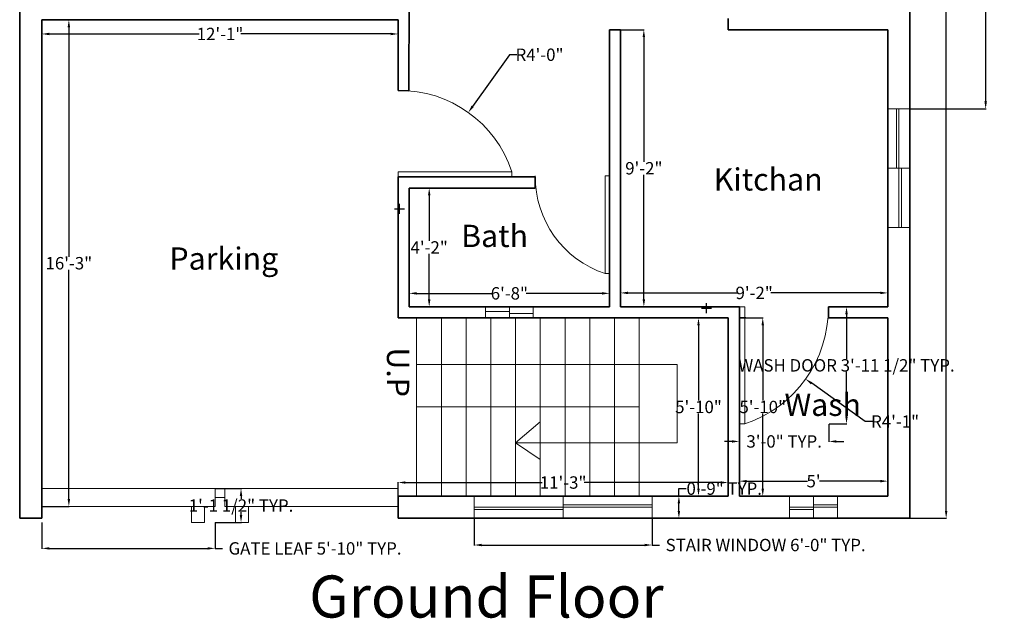
# Model space of a CAD drawing. Units: inches. Extents: x 534 to 1461, y 174 to 793.
# Tile 1 of 4: x 534 to 932, y 174 to 416. Entities that reach past the tile are written whole.
import ezdxf

# ---------------------------------------------------------------- set-up
doc = ezdxf.new("R2010")
doc.units = ezdxf.units.IN
doc.header["$MEASUREMENT"] = 0
for name, color, linetype, lineweight in [('A-ANNO-DIMS', 2, 'Continuous', 13), ('A-ANNO-SYMB', 7, 'Continuous', 15), ('A-FLOR-STRS', 7, 'Continuous', 18), ('A-GLAZ', 6, 'Continuous', 18), ('A-WALL', 7, 'Continuous', 35)]:
    doc.layers.add(name, color=color, linetype=linetype, lineweight=lineweight)
for name, color, linetype, lineweight, true_color in [('A-ANNO-TEXT', 254, 'Continuous', 18, 0xddb3d4), ('A-ANNO-TITL', 32, 'Continuous', 25, 0xcd6928), ('A-AREA-IDEN', 254, 'Continuous', 18, 0xddb3d4), ('A-DOOR', 165, 'Continuous', 20, 0x5e67af)]:
    doc.layers.add(name, color=color, linetype=linetype, lineweight=lineweight, true_color=true_color)
doc.styles.get("Standard").update_dxf_attribs({"font": 'arial.ttf'})
doc.dimstyles.get("Standard").update_dxf_attribs({"dimtxt": 5, "dimasz": 3, "dimexe": 0.18, "dimexo": 0.0625, "dimgap": 0.09, "dimtad": 0, "dimtih": 1, "dimtoh": 1, "dimdec": 1, "dimrnd": 5, "dimzin": 0, "dimdsep": 46, "dimlunit": 4, "dimtxsty": 'Standard', "dimcen": 2, "dimclrd": 4, "dimclrt": 1, "dimadec": 0, "dimazin": 0, "dimtfac": 1, "dimtdec": 1, "dimtofl": 0, "dimtmove": 0, "dimatfit": 3, "dimfxl": 1, "dimtfillclr": 1, "dimtolj": 1, "dimtzin": 0, "dimarcsym": 0})

# ---------------------------------------------------------------- blocks, each defined once
blk = doc.blocks.new('*D13')
at = {"layer": 'A-ANNO-DIMS', "color": 0, "lineweight": -2, "transparency": 16777216}
for p, q in [((691.62, 348), (699.83, 348)), ((699.65, 345), (699.65, 326.6)), ((699.65, 303), (699.65, 321.4)), ((691.62, 300), (699.83, 300))]:
    blk.add_line(p, q, dxfattribs=at)
at = {"layer": 'A-ANNO-DIMS', "color": 0, "transparency": 16777216}
for points in [[(699.15, 345), (700.15, 345), (699.65, 348)], [(699.15, 303), (700.15, 303), (699.65, 300)]]:
    blk.add_solid(points, dxfattribs=at)
at = {"layer": 'Defpoints', "color": 0, "transparency": 16777216}
for p in [(691.56, 348), (691.56, 300), (699.65, 300)]:
    blk.add_point(p, dxfattribs=at)
at = {"layer": 'A-ANNO-DIMS', "color": 0, "transparency": 16777216, "insert": (699.65, 324), "char_height": 5, "attachment_point": 5}
blk.add_mtext('\\A1;4\'-2"', dxfattribs=at)
blk = doc.blocks.new('*D14')
at = {"layer": 'A-ANNO-DIMS', "color": 0, "lineweight": -2, "transparency": 16777216}
for p, q in [((691.56, 300.06), (691.56, 305.62)), ((694.56, 305.44), (725.31, 305.44)), ((769.56, 305.44), (738.81, 305.44)), ((772.56, 300.06), (772.56, 305.62))]:
    blk.add_line(p, q, dxfattribs=at)
at = {"layer": 'A-ANNO-DIMS', "color": 0, "transparency": 16777216}
for points in [[(694.56, 305.94), (694.56, 304.94), (691.56, 305.44)], [(769.56, 305.94), (769.56, 304.94), (772.56, 305.44)]]:
    blk.add_solid(points, dxfattribs=at)
at = {"layer": 'Defpoints', "color": 0, "transparency": 16777216}
for p in [(772.56, 305.44), (691.56, 300), (772.56, 300)]:
    blk.add_point(p, dxfattribs=at)
at = {"layer": 'A-ANNO-DIMS', "color": 0, "transparency": 16777216, "insert": (732.06, 305.44), "char_height": 5, "attachment_point": 5}
blk.add_mtext('\\A1;6\'-8"', dxfattribs=at)
blk = doc.blocks.new('*D15')
at = {"layer": 'A-ANNO-DIMS', "color": 0, "lineweight": -2, "transparency": 16777216}
for p, q in [((777.12, 412), (786.62, 412)), ((786.44, 409), (786.44, 358.64)), ((786.44, 303), (786.44, 353.36)), ((777.12, 300), (786.62, 300))]:
    blk.add_line(p, q, dxfattribs=at)
at = {"layer": 'A-ANNO-DIMS', "color": 0, "transparency": 16777216}
for points in [[(785.94, 409), (786.94, 409), (786.44, 412)], [(785.94, 303), (786.94, 303), (786.44, 300)]]:
    blk.add_solid(points, dxfattribs=at)
at = {"layer": 'Defpoints', "color": 0, "transparency": 16777216}
for p in [(777.06, 412), (777.06, 300), (786.44, 300)]:
    blk.add_point(p, dxfattribs=at)
at = {"layer": 'A-ANNO-DIMS', "color": 0, "transparency": 16777216, "insert": (786.44, 356), "char_height": 5, "attachment_point": 5}
blk.add_mtext('\\A1;9\'-2"', dxfattribs=at)
blk = doc.blocks.new('*D16')
at = {"layer": 'A-ANNO-DIMS', "color": 0, "lineweight": -2, "transparency": 16777216}
for p, q in [((777.06, 300.06), (777.06, 305.79)), ((780.06, 305.61), (824.33, 305.61)), ((882.06, 305.61), (837.8, 305.61)), ((885.06, 300.06), (885.06, 305.79))]:
    blk.add_line(p, q, dxfattribs=at)
at = {"layer": 'A-ANNO-DIMS', "color": 0, "transparency": 16777216}
for points in [[(780.06, 306.11), (780.06, 305.11), (777.06, 305.61)], [(882.06, 306.11), (882.06, 305.11), (885.06, 305.61)]]:
    blk.add_solid(points, dxfattribs=at)
at = {"layer": 'Defpoints', "color": 0, "transparency": 16777216}
for p in [(885.06, 305.61), (777.06, 300), (885.06, 300)]:
    blk.add_point(p, dxfattribs=at)
at = {"layer": 'A-ANNO-DIMS', "color": 0, "transparency": 16777216, "insert": (831.06, 305.61), "char_height": 5, "attachment_point": 5}
blk.add_mtext('\\A1;9\'-2"', dxfattribs=at)
blk = doc.blocks.new('*D17')
at = {"layer": 'A-ANNO-DIMS', "color": 0, "lineweight": -2, "transparency": 16777216}
for p, q in [((825.12, 295.5), (834.7, 295.5)), ((834.52, 292.5), (834.52, 262.14)), ((834.52, 226.5), (834.52, 256.86)), ((825.12, 223.5), (834.7, 223.5))]:
    blk.add_line(p, q, dxfattribs=at)
at = {"layer": 'A-ANNO-DIMS', "color": 0, "transparency": 16777216}
for points in [[(834.02, 292.5), (835.02, 292.5), (834.52, 295.5)], [(834.02, 226.5), (835.02, 226.5), (834.52, 223.5)]]:
    blk.add_solid(points, dxfattribs=at)
at = {"layer": 'Defpoints', "color": 0, "transparency": 16777216}
for p in [(825.06, 295.5), (825.06, 223.5), (834.52, 223.5)]:
    blk.add_point(p, dxfattribs=at)
at = {"layer": 'A-ANNO-DIMS', "color": 0, "transparency": 16777216, "insert": (834.52, 259.5), "char_height": 5, "attachment_point": 5}
blk.add_mtext('\\A1;5\'-10"', dxfattribs=at)
blk = doc.blocks.new('*D18')
at = {"layer": 'A-ANNO-DIMS', "color": 0, "lineweight": -2, "transparency": 16777216}
for p, q in [((825.06, 223.56), (825.06, 229.7)), ((828.06, 229.52), (852.67, 229.52)), ((882.06, 229.52), (857.45, 229.52)), ((885.06, 223.56), (885.06, 229.7))]:
    blk.add_line(p, q, dxfattribs=at)
at = {"layer": 'A-ANNO-DIMS', "color": 0, "transparency": 16777216}
for points in [[(828.06, 230.02), (828.06, 229.02), (825.06, 229.52)], [(882.06, 230.02), (882.06, 229.02), (885.06, 229.52)]]:
    blk.add_solid(points, dxfattribs=at)
at = {"layer": 'Defpoints', "color": 0, "transparency": 16777216}
for p in [(885.06, 229.52), (825.06, 223.5), (885.06, 223.5)]:
    blk.add_point(p, dxfattribs=at)
at = {"layer": 'A-ANNO-DIMS', "color": 0, "transparency": 16777216, "insert": (855.06, 229.52), "char_height": 5, "attachment_point": 5}
blk.add_mtext("\\A1;5'", dxfattribs=at)
blk = doc.blocks.new('*D19')
at = {"layer": 'A-ANNO-DIMS', "color": 0, "lineweight": -2, "transparency": 16777216}
for p, q in [((543.12, 416), (554.12, 416)), ((553.94, 413), (553.94, 320.26)), ((553.94, 222.24), (553.94, 314.97)), ((543.12, 219.24), (554.12, 219.24))]:
    blk.add_line(p, q, dxfattribs=at)
at = {"layer": 'A-ANNO-DIMS', "color": 0, "transparency": 16777216}
for points in [[(553.44, 413), (554.44, 413), (553.94, 416)], [(553.44, 222.24), (554.44, 222.24), (553.94, 219.24)]]:
    blk.add_solid(points, dxfattribs=at)
at = {"layer": 'Defpoints', "color": 0, "transparency": 16777216}
for p in [(543.06, 416), (543.06, 219.24), (553.94, 219.24)]:
    blk.add_point(p, dxfattribs=at)
at = {"layer": 'A-ANNO-DIMS', "color": 0, "transparency": 16777216, "insert": (553.94, 317.62), "char_height": 5, "attachment_point": 5}
blk.add_mtext('\\A1;16\'-3"', dxfattribs=at)
blk = doc.blocks.new('*D20')
at = {"layer": 'A-ANNO-DIMS', "color": 0, "lineweight": -2, "transparency": 16777216}
for p, q in [((543.06, 415.94), (543.06, 410.11)), ((687.06, 415.94), (687.06, 410.11)), ((546.06, 410.29), (606.62, 410.29)), ((684.06, 410.29), (623.5, 410.29))]:
    blk.add_line(p, q, dxfattribs=at)
at = {"layer": 'A-ANNO-DIMS', "color": 0, "transparency": 16777216}
for points in [[(546.06, 410.79), (546.06, 409.79), (543.06, 410.29)], [(684.06, 410.79), (684.06, 409.79), (687.06, 410.29)]]:
    blk.add_solid(points, dxfattribs=at)
at = {"layer": 'Defpoints', "color": 0, "transparency": 16777216}
for p in [(543.06, 416), (687.06, 416), (687.06, 410.29)]:
    blk.add_point(p, dxfattribs=at)
at = {"layer": 'A-ANNO-DIMS', "color": 0, "transparency": 16777216, "insert": (615.06, 410.29), "char_height": 5, "attachment_point": 5}
blk.add_mtext('\\A1;12\'-1"', dxfattribs=at)
blk = doc.blocks.new('*D21')
at = {"layer": 'A-ANNO-DIMS', "color": 0, "lineweight": -2, "transparency": 16777216}
for p, q in [((820.5, 295.5), (808.36, 295.5)), ((808.54, 292.5), (808.54, 262.14)), ((808.54, 226.5), (808.54, 256.86)), ((820.5, 223.5), (808.36, 223.5))]:
    blk.add_line(p, q, dxfattribs=at)
at = {"layer": 'A-ANNO-DIMS', "color": 0, "transparency": 16777216}
for points in [[(808.04, 292.5), (809.04, 292.5), (808.54, 295.5)], [(808.04, 226.5), (809.04, 226.5), (808.54, 223.5)]]:
    blk.add_solid(points, dxfattribs=at)
at = {"layer": 'Defpoints', "color": 0, "transparency": 16777216}
for p in [(820.56, 295.5), (808.54, 223.5), (820.56, 223.5)]:
    blk.add_point(p, dxfattribs=at)
at = {"layer": 'A-ANNO-DIMS', "color": 0, "transparency": 16777216, "insert": (808.54, 259.5), "char_height": 5, "attachment_point": 5}
blk.add_mtext('\\A1;5\'-10"', dxfattribs=at)
blk = doc.blocks.new('*D22')
at = {"layer": 'A-ANNO-DIMS', "color": 0, "lineweight": -2, "transparency": 16777216}
for p, q in [((687.06, 223.56), (687.06, 229.14)), ((690.06, 228.96), (745.37, 228.96)), ((817.56, 228.96), (762.25, 228.96)), ((820.56, 223.56), (820.56, 229.14))]:
    blk.add_line(p, q, dxfattribs=at)
at = {"layer": 'A-ANNO-DIMS', "color": 0, "transparency": 16777216}
for points in [[(690.06, 229.46), (690.06, 228.46), (687.06, 228.96)], [(817.56, 229.46), (817.56, 228.46), (820.56, 228.96)]]:
    blk.add_solid(points, dxfattribs=at)
at = {"layer": 'Defpoints', "color": 0, "transparency": 16777216}
for p in [(820.56, 228.96), (687.06, 223.5), (820.56, 223.5)]:
    blk.add_point(p, dxfattribs=at)
at = {"layer": 'A-ANNO-DIMS', "color": 0, "transparency": 16777216, "insert": (753.81, 228.96), "char_height": 5, "attachment_point": 5}
blk.add_mtext('\\A1;11\'-3"', dxfattribs=at)
blk = doc.blocks.new('*D23')
at = {"layer": 'A-ANNO-DIMS', "color": 0, "lineweight": -2, "transparency": 16777216}
for p, q in [((894.12, 754.5), (908.87, 754.5)), ((908.69, 751.5), (908.69, 487.13)), ((908.69, 217.5), (908.69, 481.87)), ((894.12, 214.5), (908.87, 214.5))]:
    blk.add_line(p, q, dxfattribs=at)
at = {"layer": 'A-ANNO-DIMS', "color": 0, "transparency": 16777216}
for points in [[(908.19, 751.5), (909.19, 751.5), (908.69, 754.5)], [(908.19, 217.5), (909.19, 217.5), (908.69, 214.5)]]:
    blk.add_solid(points, dxfattribs=at)
at = {"layer": 'Defpoints', "color": 0, "transparency": 16777216}
for p in [(894.06, 754.5), (908.69, 754.5), (894.06, 214.5)]:
    blk.add_point(p, dxfattribs=at)
at = {"layer": 'A-ANNO-DIMS', "color": 0, "transparency": 16777216, "insert": (908.69, 484.5), "char_height": 5, "attachment_point": 5}
blk.add_mtext("\\A1;45'", dxfattribs=at)
blk = doc.blocks.new('WIN-SLIDING-48')
for p, q in [((0, 0), (0, 9)), ((24, 0), (24, 9)), ((48, 0), (48, 9)), ((0, 4.5), (48, 4.5)), ((24, 5.5), (48, 5.5)), ((0, 3.5), (24, 3.5))]:
    blk.add_line(p, q)
blk = doc.blocks.new('WIN-SLIDING-VENT-EXT')
for p, q in [((9, 19.38), (0, 19.38)), ((3.5, 19.38), (3.5, 9.69)), ((4.5, 19.38), (4.5, 0)), ((9, 9.69), (0, 9.69)), ((5.5, 9.69), (5.5, 0)), ((9, 0), (0, 0))]:
    blk.add_line(p, q)
blk = doc.blocks.new('WIN-SLIDING-VENT-STAIR')
for p, q in [((0, 0), (0, 4.5)), ((9.69, 0), (9.69, 4.5)), ((19.38, 0), (19.38, 4.5)), ((9.69, 2.58), (0, 2.58)), ((19.38, 0), (0, 0)), ((19.38, 1.76), (9.69, 1.76))]:
    blk.add_line(p, q)
blk = doc.blocks.new('WIN-SLIDING-72')
for p, q in [((0, 9), (0, 0)), ((36, 9), (36, 0)), ((72, 9), (72, 0)), ((0, 4.5), (72, 4.5)), ((36, 5.5), (72, 5.5)), ((0, 3.5), (36, 3.5))]:
    blk.add_line(p, q)
blk = doc.blocks.new('DOOR-SWING-BATH')
blk.add_lwpolyline([(30.07, 0), (28.27, 0), (28.27, 39.55), (30.07, 39.55)], close=True)
blk.add_arc((41.14, 39.08), 41.14, 179.344, 251.7744)
blk = doc.blocks.new('DOOR-SWING-ENTRY')
blk.add_lwpolyline([(45.99, 0), (45.99, 2.09), (0, 2.09), (0, 0)], close=True)
blk.add_arc((0.55, -12.87), 47.85, 18.2256, 90.656)
blk = doc.blocks.new('DOOR-SWING-WASH')
blk.add_lwpolyline([(0, 0), (2.15, 0), (2.15, 47.33), (0, 47.33)], close=True)
blk.add_arc((-13.25, 46.77), 49.24, 288.2256, 0.656)
blk = doc.blocks.new('STAIR-RETURN-FLIGHT')
for p, q in [((0, 72), (0, 0)), ((10, 72), (10, 0)), ((20, 72), (20, 0)), ((30, 72), (30, 0)), ((40, 72), (40, 0)), ((50, 72), (50, 0)), ((60, 72), (60, 0)), ((70, 72), (70, 0)), ((80, 72), (80, 0)), ((90, 72), (90, 0)), ((90, 36), (0, 36))]:
    blk.add_line(p, q)
blk = doc.blocks.new('ARROW-STAIR-RETURN')
for q in [(50, 15.21), (50, 0)]:
    blk.add_line((40, 6.74), q)
blk.add_lwpolyline([(0, 38.39), (105.42, 38.39), (105.42, 6.74), (40, 6.74)])
blk = doc.blocks.new('GATE-PARKING-LEAF')
for p, q in [((0, 13.67), (70, 13.67)), ((70, 6.41), (70, 13.67)), ((0, 6.41), (70, 6.41)), ((60.48, 0), (60.48, 6.41)), ((65.78, 6.41), (65.78, 0)), ((65.78, 0), (60.48, 0))]:
    blk.add_line(p, q)
blk = doc.blocks.new('*D71')
at = {"layer": 'A-ANNO-DIMS', "color": 0, "lineweight": -2, "transparency": 16777216}
for p, q in [((717.81, 214.44), (717.81, 203.52)), ((789.81, 214.44), (789.81, 203.52))]:
    blk.add_line(p, q, dxfattribs=at)
at = {"layer": 'A-ANNO-DIMS', "color": 4, "lineweight": -2, "transparency": 16777216}
for p, q in [((720.81, 203.7), (786.81, 203.7)), ((789.81, 203.7), (792.81, 203.7))]:
    blk.add_line(p, q, dxfattribs=at)
at = {"layer": 'A-ANNO-DIMS', "color": 4, "transparency": 16777216}
for points in [[(720.81, 204.2), (720.81, 203.2), (717.81, 203.7)], [(786.81, 204.2), (786.81, 203.2), (789.81, 203.7)]]:
    blk.add_solid(points, dxfattribs=at)
at = {"layer": 'Defpoints', "color": 0, "transparency": 16777216}
for p in [(717.81, 214.5), (789.81, 214.5), (789.81, 203.7)]:
    blk.add_point(p, dxfattribs=at)
at = {"layer": 'A-ANNO-DIMS', "color": 1, "transparency": 16777216, "insert": (835.68, 203.7), "char_height": 5, "attachment_point": 5}
blk.add_mtext('\\A1;STAIR WINDOW 6\'-0" TYP.', dxfattribs=at)
blk = doc.blocks.new('*D72')
at = {"layer": 'A-ANNO-DIMS', "color": 0, "lineweight": -2, "transparency": 16777216}
for p, q in [((789.87, 223.5), (800.79, 223.5)), ((789.87, 214.5), (800.79, 214.5))]:
    blk.add_line(p, q, dxfattribs=at)
at = {"layer": 'A-ANNO-DIMS', "color": 4, "lineweight": -2, "transparency": 16777216}
for p, q in [((800.61, 223.5), (800.61, 226.5)), ((800.61, 226.5), (803.61, 226.5)), ((800.61, 217.5), (800.61, 220.5))]:
    blk.add_line(p, q, dxfattribs=at)
at = {"layer": 'A-ANNO-DIMS', "color": 4, "transparency": 16777216}
for points in [[(800.11, 220.5), (801.11, 220.5), (800.61, 223.5)], [(800.11, 217.5), (801.11, 217.5), (800.61, 214.5)]]:
    blk.add_solid(points, dxfattribs=at)
at = {"layer": 'Defpoints', "color": 0, "transparency": 16777216}
for p in [(789.81, 223.5), (800.61, 223.5), (789.81, 214.5)]:
    blk.add_point(p, dxfattribs=at)
at = {"layer": 'A-ANNO-DIMS', "color": 1, "transparency": 16777216, "insert": (818.94, 226.5), "char_height": 5, "attachment_point": 5}
blk.add_mtext('\\A1;0\'-9" TYP.', dxfattribs=at)
blk = doc.blocks.new('*D87')
at = {"layer": 'A-ANNO-DIMS', "color": 0, "lineweight": -2, "transparency": 16777216}
for p, q in [((861.36, 300), (868.57, 300)), ((861.36, 252.67), (868.57, 252.67))]:
    blk.add_line(p, q, dxfattribs=at)
at = {"layer": 'A-ANNO-DIMS', "color": 4, "lineweight": -2, "transparency": 16777216}
for p, q in [((868.39, 297), (868.39, 279.01)), ((868.39, 255.67), (868.39, 273.66))]:
    blk.add_line(p, q, dxfattribs=at)
at = {"layer": 'A-ANNO-DIMS', "color": 4, "transparency": 16777216}
for points in [[(867.89, 297), (868.89, 297), (868.39, 300)], [(867.89, 255.67), (868.89, 255.67), (868.39, 252.67)]]:
    blk.add_solid(points, dxfattribs=at)
at = {"layer": 'Defpoints', "color": 0, "transparency": 16777216}
for p in [(861.29, 300), (868.39, 300), (861.29, 252.67)]:
    blk.add_point(p, dxfattribs=at)
at = {"layer": 'A-ANNO-DIMS', "color": 1, "transparency": 16777216, "insert": (868.39, 276.33), "char_height": 5, "attachment_point": 5}
blk.add_mtext('\\A1;WASH DOOR 3\'-11 1/2" TYP.', dxfattribs=at)
blk = doc.blocks.new('*D88')
at = {"layer": 'A-ANNO-DIMS', "color": 0, "lineweight": -2, "transparency": 16777216}
for p, q in [((825.06, 252.61), (825.06, 245.39)), ((861.29, 252.61), (861.29, 245.39))]:
    blk.add_line(p, q, dxfattribs=at)
at = {"layer": 'A-ANNO-DIMS', "color": 4, "lineweight": -2, "transparency": 16777216}
for p, q in [((822.06, 245.57), (819.06, 245.57)), ((864.29, 245.57), (867.29, 245.57))]:
    blk.add_line(p, q, dxfattribs=at)
at = {"layer": 'A-ANNO-DIMS', "color": 4, "transparency": 16777216}
for points in [[(822.06, 246.07), (822.06, 245.07), (825.06, 245.57)], [(864.29, 246.07), (864.29, 245.07), (861.29, 245.57)]]:
    blk.add_solid(points, dxfattribs=at)
at = {"layer": 'Defpoints', "color": 0, "transparency": 16777216}
for p in [(825.06, 252.67), (861.29, 252.67), (861.29, 245.57)]:
    blk.add_point(p, dxfattribs=at)
at = {"layer": 'A-ANNO-DIMS', "color": 1, "transparency": 16777216, "insert": (843.18, 245.57), "char_height": 5, "attachment_point": 5}
blk.add_mtext('\\A1;3\'-0" TYP.', dxfattribs=at)
blk = doc.blocks.new('*D89')
at = {"layer": 'A-ANNO-DIMS', "color": 0, "lineweight": -2, "transparency": 16777216}
for p, q in [((543.06, 212.76), (543.06, 202.15)), ((613.06, 212.76), (613.06, 202.15))]:
    blk.add_line(p, q, dxfattribs=at)
at = {"layer": 'A-ANNO-DIMS', "color": 4, "lineweight": -2, "transparency": 16777216}
for p, q in [((546.06, 202.33), (610.06, 202.33)), ((613.06, 202.33), (616.06, 202.33))]:
    blk.add_line(p, q, dxfattribs=at)
at = {"layer": 'A-ANNO-DIMS', "color": 4, "transparency": 16777216}
for points in [[(546.06, 202.83), (546.06, 201.83), (543.06, 202.33)], [(610.06, 202.83), (610.06, 201.83), (613.06, 202.33)]]:
    blk.add_solid(points, dxfattribs=at)
at = {"layer": 'Defpoints', "color": 0, "transparency": 16777216}
for p in [(543.06, 212.83), (613.06, 212.83), (613.06, 202.33)]:
    blk.add_point(p, dxfattribs=at)
at = {"layer": 'A-ANNO-DIMS', "color": 1, "transparency": 16777216, "insert": (653.48, 202.33), "char_height": 5, "attachment_point": 5}
blk.add_mtext('\\A1;GATE LEAF 5\'-10" TYP.', dxfattribs=at)
blk = doc.blocks.new('*D90')
at = {"layer": 'A-ANNO-DIMS', "color": 0, "lineweight": -2, "transparency": 16777216}
for p, q in [((613.12, 226.5), (623.74, 226.5)), ((613.12, 212.83), (623.74, 212.83))]:
    blk.add_line(p, q, dxfattribs=at)
at = {"layer": 'A-ANNO-DIMS', "color": 4, "lineweight": -2, "transparency": 16777216}
for p, q in [((623.56, 223.5), (623.56, 222.34)), ((623.56, 215.83), (623.56, 216.99))]:
    blk.add_line(p, q, dxfattribs=at)
at = {"layer": 'A-ANNO-DIMS', "color": 4, "transparency": 16777216}
for points in [[(623.06, 223.5), (624.06, 223.5), (623.56, 226.5)], [(623.06, 215.83), (624.06, 215.83), (623.56, 212.83)]]:
    blk.add_solid(points, dxfattribs=at)
at = {"layer": 'Defpoints', "color": 0, "transparency": 16777216}
for p in [(613.06, 226.5), (623.56, 226.5), (613.06, 212.83)]:
    blk.add_point(p, dxfattribs=at)
at = {"layer": 'A-ANNO-DIMS', "color": 1, "transparency": 16777216, "insert": (623.56, 219.66), "char_height": 5, "attachment_point": 5}
blk.add_mtext('\\A1;1\'-1 1/2" TYP.', dxfattribs=at)
blk = doc.blocks.new('*D104')
at = {"layer": 'A-ANNO-DIMS', "color": 0, "lineweight": -2, "transparency": 16777216}
for p, q in [((894.12, 482.75), (924.84, 482.75)), ((894.12, 380), (924.84, 380))]:
    blk.add_line(p, q, dxfattribs=at)
at = {"layer": 'A-ANNO-DIMS', "color": 4, "lineweight": -2, "transparency": 16777216}
for p, q in [((924.66, 479.75), (924.66, 434.02)), ((924.66, 383), (924.66, 428.73))]:
    blk.add_line(p, q, dxfattribs=at)
at = {"layer": 'A-ANNO-DIMS', "color": 4, "transparency": 16777216}
for points in [[(924.16, 479.75), (925.16, 479.75), (924.66, 482.75)], [(924.16, 383), (925.16, 383), (924.66, 380)]]:
    blk.add_solid(points, dxfattribs=at)
at = {"layer": 'Defpoints', "color": 0, "transparency": 16777216}
for p in [(894.06, 482.75), (894.06, 380), (924.66, 380)]:
    blk.add_point(p, dxfattribs=at)
at = {"layer": 'A-ANNO-DIMS', "color": 1, "transparency": 16777216, "insert": (924.66, 431.37), "char_height": 5, "attachment_point": 5}
blk.add_mtext('\\A1;8\'-7"', dxfattribs=at)
blk = doc.blocks.new('*D108')
at = {"layer": 'A-ANNO-DIMS', "color": 4, "lineweight": -2, "transparency": 16777216}
for p, q in [((732.13, 401.91), (717.18, 380.99)), ((735.13, 401.91), (732.13, 401.91))]:
    blk.add_line(p, q, dxfattribs=at)
at = {"layer": 'A-ANNO-DIMS', "color": 0, "lineweight": -2, "transparency": 16777216}
for p, q in [((685.61, 339.63), (689.61, 339.63)), ((687.61, 337.63), (687.61, 341.63))]:
    blk.add_line(p, q, dxfattribs=at)
at = {"layer": 'A-ANNO-DIMS', "color": 4, "transparency": 16777216}
blk.add_solid([(716.77, 381.28), (717.59, 380.7), (715.43, 378.55)], dxfattribs=at)
at = {"layer": 'Defpoints', "color": 0, "transparency": 16777216}
for p in [(715.43, 378.55), (687.61, 339.63)]:
    blk.add_point(p, dxfattribs=at)
at = {"layer": 'A-ANNO-DIMS', "color": 1, "transparency": 16777216, "insert": (744.26, 401.91), "char_height": 5, "attachment_point": 5}
blk.add_mtext('\\A1;R4\'-0"', dxfattribs=at)
blk = doc.blocks.new('*D112')
at = {"layer": 'A-ANNO-DIMS', "color": 0, "lineweight": -2, "transparency": 16777216}
for p, q in [((809.82, 299.44), (813.82, 299.44)), ((811.82, 297.44), (811.82, 301.44))]:
    blk.add_line(p, q, dxfattribs=at)
at = {"layer": 'A-ANNO-DIMS', "color": 4, "lineweight": -2, "transparency": 16777216}
for p, q in [((875.9, 253.62), (854.31, 269.06)), ((878.9, 253.62), (875.9, 253.62))]:
    blk.add_line(p, q, dxfattribs=at)
at = {"layer": 'A-ANNO-DIMS', "color": 4, "transparency": 16777216}
blk.add_solid([(854.6, 269.46), (854.02, 268.65), (851.87, 270.8)], dxfattribs=at)
at = {"layer": 'Defpoints', "color": 0, "transparency": 16777216}
for p in [(811.82, 299.44), (851.87, 270.8)]:
    blk.add_point(p, dxfattribs=at)
at = {"layer": 'A-ANNO-DIMS', "color": 1, "transparency": 16777216, "insert": (888.03, 253.62), "char_height": 5, "attachment_point": 5}
blk.add_mtext('\\A1;R4\'-1"', dxfattribs=at)

msp = doc.modelspace()

# ---------------------------------------------------------------- linework, layer by layer
at = {"layer": 'A-DOOR'}
msp.add_line((613.06, 222.87), (617.06, 222.87), dxfattribs=at)
at = {"layer": 'A-GLAZ'}
msp.add_line((885.06, 356), (894.06, 356), dxfattribs=at)
at = {"layer": 'A-WALL'}
for p, q in [((534.06, 214.5), (534.06, 754.5)), ((894.06, 754.5), (894.06, 214.5)), ((691.47, 387.32), (691.56, 549)), ((543.06, 214.5), (543.06, 416)), ((543.06, 416), (687.06, 416)), ((687.07, 387.47), (687.06, 416)), ((820.56, 412), (820.56, 416.5)), ((772.56, 412), (772.56, 300)), ((772.56, 412), (777.06, 412)), ((777.06, 412), (777.06, 300)), ((885.06, 412), (820.56, 412)), ((885.06, 412), (885.06, 300)), ((691.47, 387.32), (687.07, 387.47)), ((687.06, 295.5), (687.06, 352.5)), ((742.56, 352.5), (687.06, 352.5)), ((742.56, 352.5), (742.56, 348)), ((691.56, 300), (691.56, 348)), ((742.56, 348), (691.56, 348)), ((772.56, 300), (691.56, 300)), ((825.06, 300), (777.06, 300)), ((825.06, 300), (825.06, 223.5)), ((885.06, 300), (861.06, 300)), ((861.06, 300), (861.06, 295.5)), ((820.56, 295.5), (687.06, 295.5)), ((820.56, 295.5), (820.56, 223.5)), ((827.67, 295.5), (825.06, 295.5)), ((885.06, 295.5), (861.06, 295.5)), ((885.06, 295.5), (885.06, 223.5)), ((687.06, 214.5), (687.06, 223.5)), ((820.56, 223.5), (687.06, 223.5)), ((885.06, 223.5), (825.06, 223.5)), ((543.06, 214.5), (534.06, 214.5)), ((894.06, 214.5), (687.06, 214.5))]:
    msp.add_line(p, q, dxfattribs=at)

# ---------------------------------------------------------------- block references
at = {"layer": 'A-ANNO-SYMB'}
msp.add_blockref('ARROW-STAIR-RETURN', (694.56, 238.32), dxfattribs=at)
at = {"layer": 'A-DOOR'}
for name, p in [('DOOR-SWING-ENTRY', (687.06, 352.5)), ('DOOR-SWING-BATH', (742.56, 313.42)), ('DOOR-SWING-WASH', (825.06, 252.67)), ('GATE-PARKING-LEAF', (543.06, 212.83))]:
    msp.add_blockref(name, p, dxfattribs=at)
at = {"layer": 'A-DOOR', "extrusion": (0, 0, -1), "zscale": -1}
msp.add_blockref('GATE-PARKING-LEAF', (-687.06, 212.83), dxfattribs=at)
at = {"layer": 'A-FLOR-STRS'}
msp.add_blockref('STAIR-RETURN-FLIGHT', (694.56, 223.5), dxfattribs=at)
at = {"layer": 'A-GLAZ'}
for name, p, rotation in [('WIN-SLIDING-48', (885.06, 380), 270.0000000000009), ('WIN-SLIDING-VENT-EXT', (845.37, 223.5), 270.0000000000007)]:
    msp.add_blockref(name, p, dxfattribs=dict(at, rotation=rotation))
for name, p in [('WIN-SLIDING-VENT-STAIR', (722.37, 295.5)), ('WIN-SLIDING-72', (717.81, 214.5))]:
    msp.add_blockref(name, p, dxfattribs=at)

# ---------------------------------------------------------------- texts
at = {"layer": 'A-ANNO-TEXT', "insert": (691.56, 300), "char_height": 9, "attachment_point": 1, "rotation": 270}
msp.add_mtext_dynamic_manual_height_columns('\\pxqc;U.P', width=52.8697, gutter_width=1, heights=[0], dxfattribs=at)
at = {"layer": 'A-ANNO-TITL', "insert": (644.57, 191.38), "char_height": 17, "attachment_point": 1}
msp.add_mtext_dynamic_manual_height_columns('\\pxqc;Ground Floor', width=156.4181, gutter_width=1, heights=[0], dxfattribs=at)
at = {"layer": 'A-AREA-IDEN', "char_height": 9, "attachment_point": 1}
for s, insert in [('\\pxqc;Kitchan ', (810.29, 356)), ('\\pxqc;Bath', (699.65, 333.15)), ('\\pxqc;Parking ', (590.17, 324)), ('\\pxqc;Wash ', (832.34, 264.88))]:
    msp.add_mtext_dynamic_manual_height_columns(s, width=52.8697, gutter_width=1, heights=[0], dxfattribs=dict(at, insert=insert))

# ---------------------------------------------------------------- dimensions: what is measured, and where the dimension line sits
at = {"layer": 'A-ANNO-DIMS'}
for base, p1, p2, override, picture, middle in [((908.69, 754.5), (894.06, 214.5), (894.06, 754.5), {"dimclrd": 0, "dimclre": 0, "dimclrt": 0}, '*D23', (908.69, 484.5)), ((924.661818, 379.999272), (894.061818, 482.749272), (894.061818, 379.999272), {"dimdec": 1, "dimlfac": 1, "dimrnd": 0, "dimzin": 1, "dimdsep": 46, "dimlunit": 4, "dimfrac": 2}, '*D104', (924.661818, 431.374272)), ((553.94, 219.24), (543.06, 416), (543.06, 219.24), {"dimclrd": 0, "dimclre": 0, "dimclrt": 0}, '*D19', (553.94, 317.62)), ((786.44, 300), (777.06, 412), (777.06, 300), {"dimclrd": 0, "dimclre": 0, "dimclrt": 0}, '*D15', (786.44, 356)), ((699.65, 300), (691.56, 348), (691.56, 300), {"dimclrd": 0, "dimclre": 0, "dimclrt": 0}, '*D13', (699.65, 324)), ((808.54, 223.5), (820.56, 295.5), (820.56, 223.5), {"dimclrd": 0, "dimclre": 0, "dimclrt": 0}, '*D21', (808.54, 259.5)), ((834.52, 223.5), (825.06, 295.5), (825.06, 223.5), {"dimclrd": 0, "dimclre": 0, "dimclrt": 0}, '*D17', (834.52, 259.5))]:
    dim = msp.add_linear_dim(base=base, p1=p1, p2=p2, angle=90, dimstyle='Standard', override=override, dxfattribs=at)
    dim.commit()
    dim.dimension.update_dxf_attribs({"geometry": picture, "text_midpoint": middle})
for base, p1, p2, picture, middle in [((687.06, 410.29), (543.06, 416), (687.06, 416), '*D20', (615.06, 410.29)), ((772.56, 305.44), (691.56, 300), (772.56, 300), '*D14', (732.06, 305.44)), ((885.06, 305.61), (777.06, 300), (885.06, 300), '*D16', (831.06, 305.61)), ((820.56, 228.96), (687.06, 223.5), (820.56, 223.5), '*D22', (753.81, 228.96)), ((885.06, 229.52), (825.06, 223.5), (885.06, 223.5), '*D18', (855.06, 229.52))]:
    dim = msp.add_linear_dim(base=base, p1=p1, p2=p2, dimstyle='Standard', override={"dimclrd": 0, "dimclre": 0, "dimclrt": 0}, dxfattribs=at)
    dim.commit()
    dim.dimension.update_dxf_attribs({"geometry": picture, "text_midpoint": middle})
for center, mpoint, picture, middle in [((687.61, 339.63), (715.43, 378.55), '*D108', (744.26, 401.91)), ((811.82, 299.44), (851.87, 270.8), '*D112', (888.03, 253.62))]:
    dim = msp.add_radius_dim(center=center, mpoint=mpoint, dimstyle='Standard', override={"dimdec": 1, "dimlfac": 1, "dimrnd": 0, "dimzin": 1, "dimdsep": 46, "dimlunit": 4, "dimfrac": 2}, dxfattribs=at)
    dim.commit()
    dim.dimension.update_dxf_attribs({"geometry": picture, "text_midpoint": middle, "dimtype": 164})
for base, p1, p2, text, picture, middle in [((868.39, 300), (861.29, 252.67), (861.29, 300), 'WASH DOOR <> TYP.', '*D87', (868.39, 276.33)), ((623.56, 226.5), (613.06, 212.83), (613.06, 226.5), '<> TYP.', '*D90', (623.56, 219.66)), ((800.61, 223.5), (789.81, 214.5), (789.81, 223.5), '<> TYP.', '*D72', (818.94, 226.5))]:
    dim = msp.add_linear_dim(base=base, p1=p1, p2=p2, angle=90, text=text, dimstyle='Standard', override={"dimdec": 1, "dimlfac": 1, "dimrnd": 0, "dimzin": 1, "dimdsep": 46, "dimlunit": 4, "dimfrac": 2}, dxfattribs=at)
    dim.commit()
    dim.dimension.update_dxf_attribs({"geometry": picture, "text_midpoint": middle})
for base, p1, p2, text, picture, middle in [((861.29, 245.57), (825.06, 252.67), (861.29, 252.67), '<> TYP.', '*D88', (843.18, 245.57)), ((789.81, 203.7), (717.81, 214.5), (789.81, 214.5), 'STAIR WINDOW <> TYP.', '*D71', (835.68, 203.7)), ((613.06, 202.33), (543.06, 212.83), (613.06, 212.83), 'GATE LEAF <> TYP.', '*D89', (653.48, 202.33))]:
    dim = msp.add_linear_dim(base=base, p1=p1, p2=p2, text=text, dimstyle='Standard', override={"dimdec": 1, "dimlfac": 1, "dimrnd": 0, "dimzin": 1, "dimdsep": 46, "dimlunit": 4, "dimfrac": 2}, dxfattribs=at)
    dim.commit()
    dim.dimension.update_dxf_attribs({"geometry": picture, "text_midpoint": middle})

doc.saveas('drawing.dxf')
